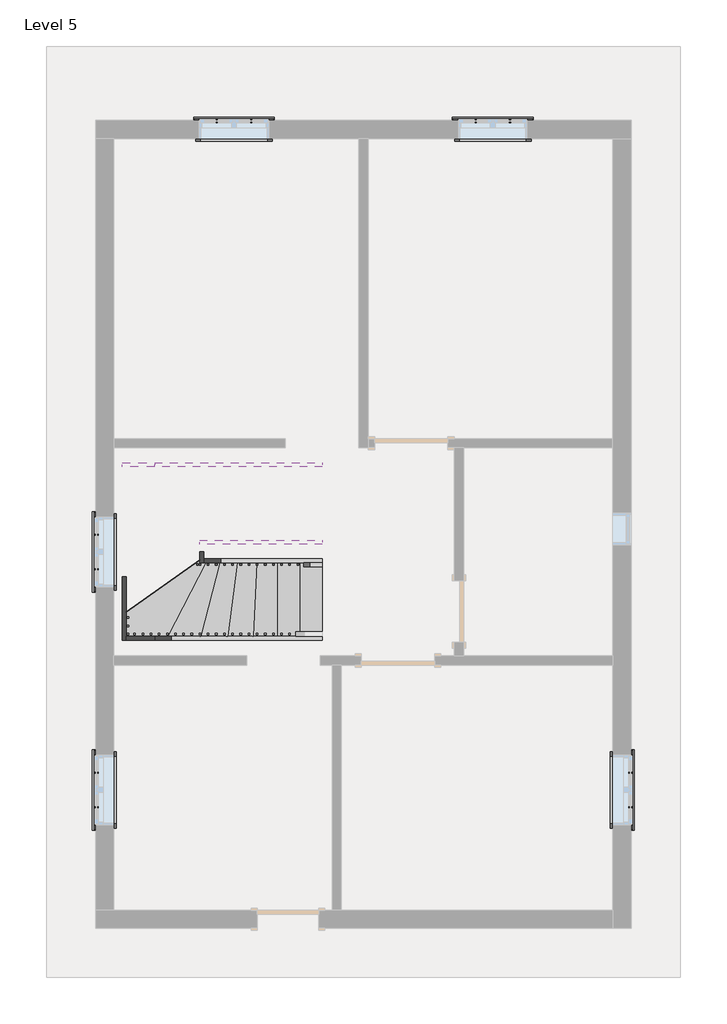
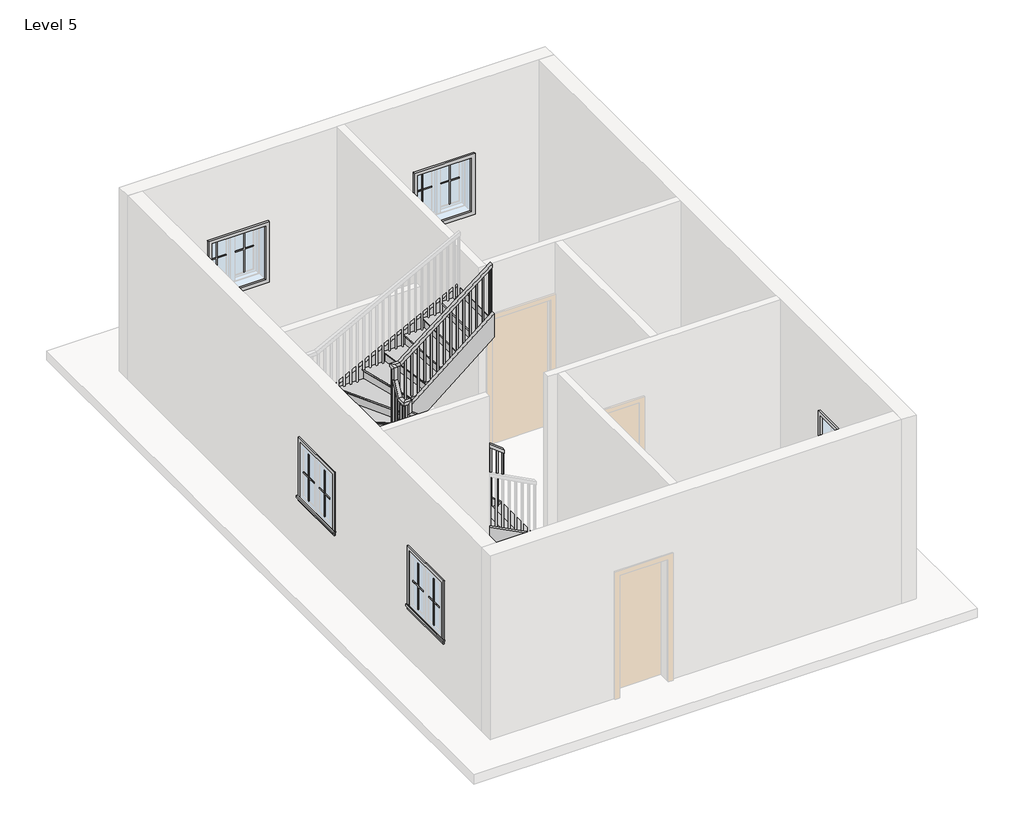
# One storey, part 2 of 2: 20 proxies, 8 members, 1 railing, 1 stair flight.
"""IFC4 building model written with IfcOpenShell, lengths in millimetres."""

from ifc_helpers import new_model, si_unit, frame, origin, place, context, project, spatial, polyline, outline, extrude, faceted_brep, transform, mapped, element, save
from components import muntin_pattern_2x2_muntin_pattern_2x2_b3fe6957, muntin_pattern_2x2_muntin_pattern_2x2_3e0ecaf2, trim_window_exterior_flat_with_sill_41619996, trim_window_interior_flat_picture_frame_51c85655, stair_flight_8889bdd5

model = new_model("IFC4")

# Units and contexts
model_context = context("Model", 3, world=origin())
ifc_project = project(units=[si_unit("LENGTHUNIT", "METRE", prefix="MILLI")], contexts=[model_context])

# Site, building, storey
site = spatial("IfcSite", under=ifc_project)
building = spatial("IfcBuilding", under=site)
storey = spatial("IfcBuildingStorey", under=building, Name="Level 5", Elevation=9601.2)

# Proxies
placement = place(None, origin())
muntin_pattern_2x2_muntin_pattern_2x2_shape = muntin_pattern_2x2_muntin_pattern_2x2_b3fe6957(model_context)
element("IfcBuildingElementProxy", 1, Name="Muntin Pattern_2x2 : Muntin Pattern_2x2", ObjectType="Muntin Pattern_2x2 : Muntin Pattern_2x2", at=placement, inside=storey, context=model_context, shape_type="MappedRepresentation", body=[
    mapped(muntin_pattern_2x2_muntin_pattern_2x2_shape, transform((-3096.8324167, 5150.2179147, 10585.45), x_axis=(1.0, 0.0, 0.0), y_axis=(0.0, 1.0, 0.0), z_axis=(0.0, 0.0, 1.0))),
])
element("IfcBuildingElementProxy", 2, Name="Muntin Pattern_2x2 : Muntin Pattern_2x2", ObjectType="Muntin Pattern_2x2 : Muntin Pattern_2x2", at=placement, inside=storey, context=model_context, shape_type="MappedRepresentation", body=[
    mapped(muntin_pattern_2x2_muntin_pattern_2x2_shape, transform((122.6175833, 5150.2179147, 10585.45), x_axis=(1.0, 0.0, 0.0), y_axis=(0.0, 1.0, 0.0), z_axis=(0.0, 0.0, 1.0))),
])
element("IfcBuildingElementProxy", 3, Name="Muntin Pattern_2x2 : Muntin Pattern_2x2", ObjectType="Muntin Pattern_2x2 : Muntin Pattern_2x2", at=placement, inside=storey, context=model_context, shape_type="MappedRepresentation", body=[
    mapped(muntin_pattern_2x2_muntin_pattern_2x2_shape, transform((2051.4300833, -2960.3195853, 10585.45), x_axis=(0.0, -1.0, 0.0), y_axis=(1.0, 0.0, 0.0), z_axis=(0.0, 0.0, 1.0))),
])
element("IfcBuildingElementProxy", 4, Name="Muntin Pattern_2x2 : Muntin Pattern_2x2", ObjectType="Muntin Pattern_2x2 : Muntin Pattern_2x2", at=placement, inside=storey, context=model_context, shape_type="MappedRepresentation", body=[
    mapped(muntin_pattern_2x2_muntin_pattern_2x2_shape, transform((-4597.0199167, -3388.9445853, 10585.45), x_axis=(0.0, 1.0, 0.0), y_axis=(-1.0, 0.0, 0.0), z_axis=(0.0, 0.0, 1.0))),
])
element("IfcBuildingElementProxy", 5, Name="Muntin Pattern_2x2 : Muntin Pattern_2x2", ObjectType="Muntin Pattern_2x2 : Muntin Pattern_2x2", at=placement, inside=storey, context=model_context, shape_type="MappedRepresentation", body=[
    mapped(muntin_pattern_2x2_muntin_pattern_2x2_shape, transform((-4597.0199167, -426.6695853, 10585.45), x_axis=(0.0, 1.0, 0.0), y_axis=(-1.0, 0.0, 0.0), z_axis=(0.0, 0.0, 1.0))),
])
muntin_pattern_2x2_muntin_pattern_2x2_2_shape = muntin_pattern_2x2_muntin_pattern_2x2_3e0ecaf2(model_context)
element("IfcBuildingElementProxy", 6, Name="Muntin Pattern_2x2 : Muntin Pattern_2x2", ObjectType="Muntin Pattern_2x2 : Muntin Pattern_2x2", at=placement, inside=storey, context=model_context, shape_type="MappedRepresentation", body=[
    mapped(muntin_pattern_2x2_muntin_pattern_2x2_2_shape, transform((-2668.2074167, 5150.2179147, 10585.45), x_axis=(-1.0, 0.0, 0.0), y_axis=(0.0, -1.0, 0.0), z_axis=(0.0, 0.0, 1.0))),
])
element("IfcBuildingElementProxy", 7, Name="Muntin Pattern_2x2 : Muntin Pattern_2x2", ObjectType="Muntin Pattern_2x2 : Muntin Pattern_2x2", at=placement, inside=storey, context=model_context, shape_type="MappedRepresentation", body=[
    mapped(muntin_pattern_2x2_muntin_pattern_2x2_2_shape, transform((551.2425833, 5150.2179147, 10585.45), x_axis=(-1.0, 0.0, 0.0), y_axis=(0.0, -1.0, 0.0), z_axis=(0.0, 0.0, 1.0))),
])
element("IfcBuildingElementProxy", 8, Name="Muntin Pattern_2x2 : Muntin Pattern_2x2", ObjectType="Muntin Pattern_2x2 : Muntin Pattern_2x2", at=placement, inside=storey, context=model_context, shape_type="MappedRepresentation", body=[
    mapped(muntin_pattern_2x2_muntin_pattern_2x2_2_shape, transform((2051.4300833, -3388.9445853, 10585.45), x_axis=(0.0, 1.0, 0.0), y_axis=(-1.0, 0.0, 0.0), z_axis=(0.0, 0.0, 1.0))),
])
element("IfcBuildingElementProxy", 9, Name="Muntin Pattern_2x2 : Muntin Pattern_2x2", ObjectType="Muntin Pattern_2x2 : Muntin Pattern_2x2", at=placement, inside=storey, context=model_context, shape_type="MappedRepresentation", body=[
    mapped(muntin_pattern_2x2_muntin_pattern_2x2_2_shape, transform((-4597.0199167, -2960.3195853, 10585.45), x_axis=(0.0, -1.0, 0.0), y_axis=(1.0, 0.0, 0.0), z_axis=(0.0, 0.0, 1.0))),
])
element("IfcBuildingElementProxy", 10, Name="Muntin Pattern_2x2 : Muntin Pattern_2x2", ObjectType="Muntin Pattern_2x2 : Muntin Pattern_2x2", at=placement, inside=storey, context=model_context, shape_type="MappedRepresentation", body=[
    mapped(muntin_pattern_2x2_muntin_pattern_2x2_2_shape, transform((-4597.0199167, 1.9554147, 10585.45), x_axis=(0.0, -1.0, 0.0), y_axis=(1.0, 0.0, 0.0), z_axis=(0.0, 0.0, 1.0))),
])
trim_window_exterior_flat_with_sill_shape = trim_window_exterior_flat_with_sill_41619996(model_context)
element("IfcBuildingElementProxy", 11, Name="Trim-Window-Exterior-Flat : with Sill", ObjectType="Trim-Window-Exterior-Flat : with Sill", at=placement, inside=storey, context=model_context, shape_type="MappedRepresentation", body=[
    mapped(trim_window_exterior_flat_with_sill_shape, transform((-2882.5199167, 5159.7429147, 11430.0), x_axis=(-1.0, 0.0, 0.0), y_axis=(0.0, 0.0, 1.0), z_axis=(0.0, 1.0, 0.0))),
])
element("IfcBuildingElementProxy", 12, Name="Trim-Window-Exterior-Flat : with Sill", ObjectType="Trim-Window-Exterior-Flat : with Sill", at=placement, inside=storey, context=model_context, shape_type="MappedRepresentation", body=[
    mapped(trim_window_exterior_flat_with_sill_shape, transform((336.9300833, 5159.7429147, 11430.0), x_axis=(-1.0, 0.0, 0.0), y_axis=(0.0, 0.0, 1.0), z_axis=(0.0, 1.0, 0.0))),
])
element("IfcBuildingElementProxy", 13, Name="Trim-Window-Exterior-Flat : with Sill", ObjectType="Trim-Window-Exterior-Flat : with Sill", at=placement, inside=storey, context=model_context, shape_type="MappedRepresentation", body=[
    mapped(trim_window_exterior_flat_with_sill_shape, transform((2060.9550833, -3174.6320853, 11430.0), x_axis=(0.0, 1.0, 0.0), y_axis=(0.0, 0.0, 1.0), z_axis=(1.0, 0.0, 0.0))),
])
element("IfcBuildingElementProxy", 14, Name="Trim-Window-Exterior-Flat : with Sill", ObjectType="Trim-Window-Exterior-Flat : with Sill", at=placement, inside=storey, context=model_context, shape_type="MappedRepresentation", body=[
    mapped(trim_window_exterior_flat_with_sill_shape, transform((-4606.5449167, -3174.6320853, 11430.0), x_axis=(0.0, -1.0, 0.0), y_axis=(0.0, 0.0, 1.0), z_axis=(-1.0, 0.0, 0.0))),
])
element("IfcBuildingElementProxy", 15, Name="Trim-Window-Exterior-Flat : with Sill", ObjectType="Trim-Window-Exterior-Flat : with Sill", at=placement, inside=storey, context=model_context, shape_type="MappedRepresentation", body=[
    mapped(trim_window_exterior_flat_with_sill_shape, transform((-4606.5449167, -212.3570853, 11430.0), x_axis=(0.0, -1.0, 0.0), y_axis=(0.0, 0.0, 1.0), z_axis=(-1.0, 0.0, 0.0))),
])
trim_window_interior_flat_picture_frame_shape = trim_window_interior_flat_picture_frame_51c85655(model_context)
element("IfcBuildingElementProxy", 16, Name="Trim-Window-Interior-Flat : Picture Frame", ObjectType="Trim-Window-Interior-Flat : Picture Frame", at=placement, inside=storey, context=model_context, shape_type="MappedRepresentation", body=[
    mapped(trim_window_interior_flat_picture_frame_shape, transform((-2882.5199167, 4931.1429147, 11430.0), x_axis=(1.0, 0.0, 0.0), y_axis=(0.0, 0.0, 1.0), z_axis=(0.0, -1.0, 0.0))),
])
element("IfcBuildingElementProxy", 17, Name="Trim-Window-Interior-Flat : Picture Frame", ObjectType="Trim-Window-Interior-Flat : Picture Frame", at=placement, inside=storey, context=model_context, shape_type="MappedRepresentation", body=[
    mapped(trim_window_interior_flat_picture_frame_shape, transform((336.9300833, 4931.1429147, 11430.0), x_axis=(1.0, 0.0, 0.0), y_axis=(0.0, 0.0, 1.0), z_axis=(0.0, -1.0, 0.0))),
])
element("IfcBuildingElementProxy", 18, Name="Trim-Window-Interior-Flat : Picture Frame", ObjectType="Trim-Window-Interior-Flat : Picture Frame", at=placement, inside=storey, context=model_context, shape_type="MappedRepresentation", body=[
    mapped(trim_window_interior_flat_picture_frame_shape, transform((1832.3550833, -3174.6320853, 11430.0), x_axis=(0.0, -1.0, 0.0), y_axis=(0.0, 0.0, 1.0), z_axis=(-1.0, 0.0, 0.0))),
])
element("IfcBuildingElementProxy", 19, Name="Trim-Window-Interior-Flat : Picture Frame", ObjectType="Trim-Window-Interior-Flat : Picture Frame", at=placement, inside=storey, context=model_context, shape_type="MappedRepresentation", body=[
    mapped(trim_window_interior_flat_picture_frame_shape, transform((-4377.9449167, -3174.6320853, 11430.0), x_axis=(0.0, 1.0, 0.0), y_axis=(0.0, 0.0, 1.0), z_axis=(1.0, 0.0, 0.0))),
])
element("IfcBuildingElementProxy", 20, Name="Trim-Window-Interior-Flat : Picture Frame", ObjectType="Trim-Window-Interior-Flat : Picture Frame", at=placement, inside=storey, context=model_context, shape_type="MappedRepresentation", body=[
    mapped(trim_window_interior_flat_picture_frame_shape, transform((-4377.9449167, -212.3570853, 11430.0), x_axis=(0.0, 1.0, 0.0), y_axis=(0.0, 0.0, 1.0), z_axis=(1.0, 0.0, 0.0))),
])

# Members
element("IfcMember", 21, ObjectType="Stringer - 2\" Width", at=placement, inside=storey, context=model_context, shape_type="SweptSolid", body=[
    extrude(outline(polyline([(9601.2, -1783.4132248), (9830.839954, -1783.4132248), (10906.5956453, -3870.8304165), (10563.700629, -3870.8304165), (9601.2, -2003.1755424), (9601.2, -1783.4132248)])), frame((0.0, -1310.9070853, 0.0), z_axis=(0.0, 1.0, 0.0), x_axis=(0.0, 0.0, 1.0)), (0.0, 0.0, 1.0), 50.8),
])
element("IfcMember", 22, ObjectType="Stringer - 2\" Width", at=placement, inside=storey, context=model_context, shape_type="SweptSolid", body=[
    extrude(outline(polyline([(-3870.8304165, -1260.1070853), (-3870.8304165, -1310.9070853), (-4225.5449167, -1310.9070853), (-4225.5449167, -1260.1070853), (-3870.8304165, -1260.1070853)])), frame((0.0, 0.0, 10563.700629), z_axis=(0.0, 0.0, 1.0), x_axis=(1.0, 0.0, 0.0)), (0.0, 0.0, 1.0), 342.8950162),
])
element("IfcMember", 23, ObjectType="Stringer - 2\" Width", at=placement, inside=storey, context=model_context, shape_type="SweptSolid", body=[
    extrude(outline(polyline([(-1310.9070853, 10601.7956453), (-1310.9070853, 10890.2952212), (811.1127974, 11571.1972697), (848.0929147, 11571.1972697), (848.0929147, 11240.1682298), (-1141.3846024, 10601.7956453), (-1310.9070853, 10601.7956453)])), frame((-4276.3449167, 0.0, 0.0), z_axis=(1.0, 0.0, 0.0), x_axis=(0.0, 1.0, 0.0)), (0.0, 0.0, 1.0), 50.8),
])
element("IfcMember", 24, ObjectType="Stringer - 2\" Width", at=placement, inside=storey, context=model_context, shape_type="SweptSolid", body=[
    extrude(outline(polyline([(-4276.3449167, 848.0929147), (-4276.3449167, 898.8929147), (-3870.8304165, 898.8929147), (-3870.8304165, 848.0929147), (-4276.3449167, 848.0929147)])), frame((0.0, 0.0, 11251.0904473), z_axis=(0.0, 0.0, 1.0), x_axis=(1.0, 0.0, 0.0)), (0.0, 0.0, 1.0), 320.1068224),
])
element("IfcMember", 25, ObjectType="Stringer - 2\" Width", at=placement, inside=storey, context=model_context, shape_type="SweptSolid", body=[
    extrude(outline(polyline([(11571.1972697, -3870.8304165), (11251.0904473, -3870.8304165), (12326.8461385, -1783.4132248), (12646.9529609, -1783.4132248), (11571.1972697, -3870.8304165)])), frame((0.0, 848.0929147, 0.0), z_axis=(0.0, 1.0, 0.0), x_axis=(0.0, 0.0, 1.0)), (0.0, 0.0, 1.0), 50.8),
])
element("IfcMember", 26, ObjectType="Stringer - 2\" Width", at=placement, inside=storey, context=model_context, shape_type="SweptSolid", body=[
    extrude(outline(polyline([(9601.2, -1783.4132248), (9777.3764461, -1783.4132248), (10981.618648, -3260.3449167), (10588.3410923, -3260.3449167), (9601.2, -2049.6748694), (9601.2, -1783.4132248)])), frame((0.0, -345.7070853, 0.0), z_axis=(0.0, 1.0, 0.0), x_axis=(0.0, 0.0, 1.0)), (0.0, 0.0, 1.0), 50.8),
])
element("IfcMember", 27, ObjectType="Stringer - 2\" Width", at=placement, inside=storey, context=model_context, shape_type="SweptSolid", body=[
    extrude(outline(polyline([(-345.7070853, 10629.7617647), (-345.7070853, 11174.4682978), (-139.0699679, 11527.3409689), (-117.1070853, 11527.3409689), (-117.1070853, 10961.665107), (-311.464868, 10629.7617647), (-345.7070853, 10629.7617647)])), frame((-3311.1449167, 0.0, 0.0), z_axis=(1.0, 0.0, 0.0), x_axis=(0.0, 1.0, 0.0)), (0.0, 0.0, 1.0), 50.8),
])
element("IfcMember", 28, ObjectType="Stringer - 2\" Width", at=placement, inside=storey, context=model_context, shape_type="SweptSolid", body=[
    extrude(outline(polyline([(11527.3409689, -3311.1449167), (11134.0634131, -3311.1449167), (12379.7262875, -1783.4132248), (12773.0038432, -1783.4132248), (11527.3409689, -3311.1449167)])), frame((0.0, -117.1070853, 0.0), z_axis=(0.0, 1.0, 0.0), x_axis=(0.0, 0.0, 1.0)), (0.0, 0.0, 1.0), 50.8),
])

# Railing
element("IfcRailing", 29, ObjectType="Handrail - Rectangular", at=placement, inside=storey, context=model_context, shape_type="SolidModel", body=[
    faceted_brep([(-1783.4132248, -396.5070853, 10684.9333333), (-1783.4132248, -396.5070853, 10620.6000346), (-1783.4132248, -345.7070853, 10620.6000346), (-1783.4132248, -345.7070853, 10684.9333333), (-3234.9449167, -396.5070853, 11812.8191036), (-3285.7449167, -396.5070853, 11787.9590024), (-3285.7449167, -345.7070853, 11787.9590024), (-3234.9449167, -345.7070853, 11812.8191036), (-3234.9449167, -396.5070853, 12015.8281882), (-3285.7449167, -396.5070853, 11965.0281882), (-3285.7449167, -345.7070853, 11965.0281882), (-3234.9449167, -345.7070853, 12015.8281882), (-3361.9449167, -396.5070853, 12015.8281882), (-3361.9449167, -396.5070853, 11965.0281882), (-3311.1449167, -345.7070853, 11965.0281882), (-3311.1449167, -345.7070853, 12015.8281882), (-3361.9449167, -269.5070853, 12015.8281882), (-3361.9449167, -240.3857515, 11965.0281882), (-3311.1449167, -240.3857515, 11965.0281882), (-3311.1449167, -269.5070853, 12015.8281882), (-3361.9449167, -142.5070853, 12232.7051451), (-3361.9449167, -91.7070853, 12218.9256424), (-3311.1449167, -91.7070853, 12218.9256424), (-3311.1449167, -142.5070853, 12232.7051451), (-3361.9449167, -142.5070853, 12435.7142297), (-3361.9449167, -91.7070853, 12384.9142297), (-3311.1449167, -91.7070853, 12384.9142297), (-3311.1449167, -142.5070853, 12435.7142297), (-3361.9449167, -15.5070853, 12435.7142297), (-3361.9449167, -15.5070853, 12384.9142297), (-3311.1449167, -66.3070853, 12384.9142297), (-3311.1449167, -66.3070853, 12435.7142297), (-3234.9449167, -15.5070853, 12435.7142297), (-3217.5282487, -15.5070853, 12384.9142297), (-3217.5282487, -66.3070853, 12384.9142297), (-3234.9449167, -66.3070853, 12435.7142297), (-1783.4132248, -15.5070853, 13563.6), (-1783.4132248, -66.3070853, 13563.6), (-1783.4132248, -66.3070853, 13499.2667013), (-1783.4132248, -15.5070853, 13499.2667013)], [[[0, 1, 2, 3]], [[1, 0, 4, 5]], [[2, 1, 5, 6]], [[3, 2, 6, 7]], [[0, 3, 7, 4]], [[5, 4, 8, 9]], [[6, 5, 9, 10]], [[7, 6, 10, 11]], [[4, 7, 11, 8]], [[9, 8, 12, 13]], [[10, 9, 13, 14]], [[11, 10, 14, 15]], [[8, 11, 15, 12]], [[13, 12, 16, 17]], [[14, 13, 17, 18]], [[15, 14, 18, 19]], [[12, 15, 19, 16]], [[17, 16, 20, 21]], [[18, 17, 21, 22]], [[19, 18, 22, 23]], [[16, 19, 23, 20]], [[21, 20, 24, 25]], [[22, 21, 25, 26]], [[23, 22, 26, 27]], [[20, 23, 27, 24]], [[25, 24, 28, 29]], [[26, 25, 29, 30]], [[27, 26, 30, 31]], [[24, 27, 31, 28]], [[29, 28, 32, 33]], [[30, 29, 33, 34]], [[31, 30, 34, 35]], [[28, 31, 35, 32]], [[36, 37, 38, 39]], [[33, 32, 36, 39]], [[34, 33, 39, 38]], [[35, 34, 38, 37]], [[32, 35, 37, 36]]]),
    extrude(outline(polyline([(13484.0316852, -1803.0199167), (13469.2292361, -1822.0699167), (12479.8666667, -1822.0699167), (12479.8666667, -1803.0199167), (13484.0316852, -1803.0199167)])), frame((0.0, -50.4320853, 0.0), z_axis=(0.0, 1.0, 0.0), x_axis=(0.0, 0.0, 1.0)), (0.0, 0.0, 1.0), 19.05),
    extrude(outline(polyline([(13405.0852902, -1904.6199167), (13390.2828411, -1923.6699167), (12479.8666667, -1923.6699167), (12479.8666667, -1904.6199167), (13405.0852902, -1904.6199167)])), frame((0.0, -50.4320853, 0.0), z_axis=(0.0, 1.0, 0.0), x_axis=(0.0, 0.0, 1.0)), (0.0, 0.0, 1.0), 19.05),
    extrude(outline(polyline([(13326.1388952, -2006.2199167), (13311.3364462, -2025.2699167), (12479.8666667, -2025.2699167), (12479.8666667, -2006.2199167), (13326.1388952, -2006.2199167)])), frame((0.0, -50.4320853, 0.0), z_axis=(0.0, 1.0, 0.0), x_axis=(0.0, 0.0, 1.0)), (0.0, 0.0, 1.0), 19.05),
    extrude(outline(polyline([(13247.1925003, -2107.8199167), (13232.3900512, -2126.8699167), (12310.5333333, -2126.8699167), (12310.5333333, -2107.8199167), (13247.1925003, -2107.8199167)])), frame((0.0, -50.4320853, 0.0), z_axis=(0.0, 1.0, 0.0), x_axis=(0.0, 0.0, 1.0)), (0.0, 0.0, 1.0), 19.05),
    extrude(outline(polyline([(13168.2461053, -2209.4199167), (13153.4436562, -2228.4699167), (12310.5333333, -2228.4699167), (12310.5333333, -2209.4199167), (13168.2461053, -2209.4199167)])), frame((0.0, -50.4320853, 0.0), z_axis=(0.0, 1.0, 0.0), x_axis=(0.0, 0.0, 1.0)), (0.0, 0.0, 1.0), 19.05),
    extrude(outline(polyline([(13089.2997103, -2311.0199167), (13074.4972613, -2330.0699167), (12310.5333333, -2330.0699167), (12310.5333333, -2311.0199167), (13089.2997103, -2311.0199167)])), frame((0.0, -50.4320853, 0.0), z_axis=(0.0, 1.0, 0.0), x_axis=(0.0, 0.0, 1.0)), (0.0, 0.0, 1.0), 19.05),
    extrude(outline(polyline([(13010.3533154, -2412.6199167), (12995.5508663, -2431.6699167), (12141.2, -2431.6699167), (12141.2, -2412.6199167), (13010.3533154, -2412.6199167)])), frame((0.0, -50.4320853, 0.0), z_axis=(0.0, 1.0, 0.0), x_axis=(0.0, 0.0, 1.0)), (0.0, 0.0, 1.0), 19.05),
    extrude(outline(polyline([(12931.4069204, -2514.2199167), (12916.6044713, -2533.2699167), (12141.2, -2533.2699167), (12141.2, -2514.2199167), (12931.4069204, -2514.2199167)])), frame((0.0, -50.4320853, 0.0), z_axis=(0.0, 1.0, 0.0), x_axis=(0.0, 0.0, 1.0)), (0.0, 0.0, 1.0), 19.05),
    extrude(outline(polyline([(12852.4605254, -2615.8199167), (12837.6580764, -2634.8699167), (11971.8666667, -2634.8699167), (11971.8666667, -2615.8199167), (12852.4605254, -2615.8199167)])), frame((0.0, -50.4320853, 0.0), z_axis=(0.0, 1.0, 0.0), x_axis=(0.0, 0.0, 1.0)), (0.0, 0.0, 1.0), 19.05),
    extrude(outline(polyline([(12773.5141304, -2717.4199167), (12758.7116814, -2736.4699167), (11971.8666667, -2736.4699167), (11971.8666667, -2717.4199167), (12773.5141304, -2717.4199167)])), frame((0.0, -50.4320853, 0.0), z_axis=(0.0, 1.0, 0.0), x_axis=(0.0, 0.0, 1.0)), (0.0, 0.0, 1.0), 19.05),
    extrude(outline(polyline([(12694.5677355, -2819.0199167), (12679.7652864, -2838.0699167), (11971.8666667, -2838.0699167), (11971.8666667, -2819.0199167), (12694.5677355, -2819.0199167)])), frame((0.0, -50.4320853, 0.0), z_axis=(0.0, 1.0, 0.0), x_axis=(0.0, 0.0, 1.0)), (0.0, 0.0, 1.0), 19.05),
    extrude(outline(polyline([(12615.6213405, -2920.6199167), (12600.8188914, -2939.6699167), (11802.5333333, -2939.6699167), (11802.5333333, -2920.6199167), (12615.6213405, -2920.6199167)])), frame((0.0, -50.4320853, 0.0), z_axis=(0.0, 1.0, 0.0), x_axis=(0.0, 0.0, 1.0)), (0.0, 0.0, 1.0), 19.05),
    extrude(outline(polyline([(12536.6749455, -3022.2199167), (12521.8724965, -3041.2699167), (11802.5333333, -3041.2699167), (11802.5333333, -3022.2199167), (12536.6749455, -3022.2199167)])), frame((0.0, -50.4320853, 0.0), z_axis=(0.0, 1.0, 0.0), x_axis=(0.0, 0.0, 1.0)), (0.0, 0.0, 1.0), 19.05),
    extrude(outline(polyline([(12457.7285506, -3123.8199167), (12442.9261015, -3142.8699167), (11633.2, -3142.8699167), (11633.2, -3123.8199167), (12457.7285506, -3123.8199167)])), frame((0.0, -50.4320853, 0.0), z_axis=(0.0, 1.0, 0.0), x_axis=(0.0, 0.0, 1.0)), (0.0, 0.0, 1.0), 19.05),
    extrude(outline(polyline([(12378.7821556, -3225.4199167), (12363.9797065, -3244.4699167), (11633.2, -3244.4699167), (11633.2, -3225.4199167), (12378.7821556, -3225.4199167)])), frame((0.0, -50.4320853, 0.0), z_axis=(0.0, 1.0, 0.0), x_axis=(0.0, 0.0, 1.0)), (0.0, 0.0, 1.0), 19.05),
    extrude(outline(polyline([(-3327.0199167, -75.8320853), (-3346.0699167, -75.8320853), (-3346.0699167, -56.7820853), (-3327.0199167, -56.7820853), (-3327.0199167, -75.8320853)])), frame((0.0, 0.0, 11294.5333333), z_axis=(0.0, 0.0, 1.0), x_axis=(1.0, 0.0, 0.0)), (0.0, 0.0, 1.0), 1090.3808964),
    extrude(outline(polyline([(-177.4320853, 12072.5336964), (-158.3820853, 12105.06524), (-158.3820853, 11125.2), (-177.4320853, 11125.2), (-177.4320853, 12072.5336964)])), frame((-3346.0699167, 0.0, 0.0), z_axis=(1.0, 0.0, 0.0), x_axis=(0.0, 1.0, 0.0)), (0.0, 0.0, 1.0), 19.05),
    extrude(outline(polyline([(-279.0320853, 11899.0321309), (-259.9820853, 11931.5636744), (-259.9820853, 10955.8666667), (-279.0320853, 10955.8666667), (-279.0320853, 11899.0321309)])), frame((-3346.0699167, 0.0, 0.0), z_axis=(1.0, 0.0, 0.0), x_axis=(0.0, 1.0, 0.0)), (0.0, 0.0, 1.0), 19.05),
    extrude(outline(polyline([(-3297.8882248, -361.5820853), (-3297.8882248, -380.6320853), (-3316.9382248, -380.6320853), (-3316.9382248, -361.5820853), (-3297.8882248, -361.5820853)])), frame((0.0, 0.0, 10786.5333333), z_axis=(0.0, 0.0, 1.0), x_axis=(1.0, 0.0, 0.0)), (0.0, 0.0, 1.0), 1178.4948549),
    extrude(outline(polyline([(11718.4483397, -3196.2882248), (11733.2507888, -3215.3382248), (10617.2, -3215.3382248), (10617.2, -3196.2882248), (11718.4483397, -3196.2882248)])), frame((0.0, -380.6320853, 0.0), z_axis=(0.0, 1.0, 0.0), x_axis=(0.0, 0.0, 1.0)), (0.0, 0.0, 1.0), 19.05),
    extrude(outline(polyline([(11639.5019447, -3094.6882248), (11654.3043938, -3113.7382248), (10617.2, -3113.7382248), (10617.2, -3094.6882248), (11639.5019447, -3094.6882248)])), frame((0.0, -380.6320853, 0.0), z_axis=(0.0, 1.0, 0.0), x_axis=(0.0, 0.0, 1.0)), (0.0, 0.0, 1.0), 19.05),
    extrude(outline(polyline([(11560.5555498, -2993.0882248), (11575.3579988, -3012.1382248), (10447.8666667, -3012.1382248), (10447.8666667, -2993.0882248), (11560.5555498, -2993.0882248)])), frame((0.0, -380.6320853, 0.0), z_axis=(0.0, 1.0, 0.0), x_axis=(0.0, 0.0, 1.0)), (0.0, 0.0, 1.0), 19.05),
    extrude(outline(polyline([(11481.6091548, -2891.4882248), (11496.4116039, -2910.5382248), (10447.8666667, -2910.5382248), (10447.8666667, -2891.4882248), (11481.6091548, -2891.4882248)])), frame((0.0, -380.6320853, 0.0), z_axis=(0.0, 1.0, 0.0), x_axis=(0.0, 0.0, 1.0)), (0.0, 0.0, 1.0), 19.05),
    extrude(outline(polyline([(11402.6627598, -2789.8882248), (11417.4652089, -2808.9382248), (10278.5333333, -2808.9382248), (10278.5333333, -2789.8882248), (11402.6627598, -2789.8882248)])), frame((0.0, -380.6320853, 0.0), z_axis=(0.0, 1.0, 0.0), x_axis=(0.0, 0.0, 1.0)), (0.0, 0.0, 1.0), 19.05),
    extrude(outline(polyline([(11323.7163649, -2688.2882248), (11338.5188139, -2707.3382248), (10278.5333333, -2707.3382248), (10278.5333333, -2688.2882248), (11323.7163649, -2688.2882248)])), frame((0.0, -380.6320853, 0.0), z_axis=(0.0, 1.0, 0.0), x_axis=(0.0, 0.0, 1.0)), (0.0, 0.0, 1.0), 19.05),
    extrude(outline(polyline([(11244.7699699, -2586.6882248), (11259.5724189, -2605.7382248), (10109.2, -2605.7382248), (10109.2, -2586.6882248), (11244.7699699, -2586.6882248)])), frame((0.0, -380.6320853, 0.0), z_axis=(0.0, 1.0, 0.0), x_axis=(0.0, 0.0, 1.0)), (0.0, 0.0, 1.0), 19.05),
    extrude(outline(polyline([(11165.8235749, -2485.0882248), (11180.626024, -2504.1382248), (10109.2, -2504.1382248), (10109.2, -2485.0882248), (11165.8235749, -2485.0882248)])), frame((0.0, -380.6320853, 0.0), z_axis=(0.0, 1.0, 0.0), x_axis=(0.0, 0.0, 1.0)), (0.0, 0.0, 1.0), 19.05),
    extrude(outline(polyline([(11086.8771799, -2383.4882248), (11101.679629, -2402.5382248), (10109.2, -2402.5382248), (10109.2, -2383.4882248), (11086.8771799, -2383.4882248)])), frame((0.0, -380.6320853, 0.0), z_axis=(0.0, 1.0, 0.0), x_axis=(0.0, 0.0, 1.0)), (0.0, 0.0, 1.0), 19.05),
    extrude(outline(polyline([(11007.930785, -2281.8882248), (11022.733234, -2300.9382248), (9939.8666667, -2300.9382248), (9939.8666667, -2281.8882248), (11007.930785, -2281.8882248)])), frame((0.0, -380.6320853, 0.0), z_axis=(0.0, 1.0, 0.0), x_axis=(0.0, 0.0, 1.0)), (0.0, 0.0, 1.0), 19.05),
    extrude(outline(polyline([(10928.98439, -2180.2882248), (10943.7868391, -2199.3382248), (9939.8666667, -2199.3382248), (9939.8666667, -2180.2882248), (10928.98439, -2180.2882248)])), frame((0.0, -380.6320853, 0.0), z_axis=(0.0, 1.0, 0.0), x_axis=(0.0, 0.0, 1.0)), (0.0, 0.0, 1.0), 19.05),
    extrude(outline(polyline([(10850.037995, -2078.6882248), (10864.8404441, -2097.7382248), (9939.8666667, -2097.7382248), (9939.8666667, -2078.6882248), (10850.037995, -2078.6882248)])), frame((0.0, -380.6320853, 0.0), z_axis=(0.0, 1.0, 0.0), x_axis=(0.0, 0.0, 1.0)), (0.0, 0.0, 1.0), 19.05),
    extrude(outline(polyline([(10771.0916001, -1977.0882248), (10785.8940491, -1996.1382248), (9770.5333333, -1996.1382248), (9770.5333333, -1977.0882248), (10771.0916001, -1977.0882248)])), frame((0.0, -380.6320853, 0.0), z_axis=(0.0, 1.0, 0.0), x_axis=(0.0, 0.0, 1.0)), (0.0, 0.0, 1.0), 19.05),
    extrude(outline(polyline([(10692.1452051, -1875.4882248), (10706.9476541, -1894.5382248), (9770.5333333, -1894.5382248), (9770.5333333, -1875.4882248), (10692.1452051, -1875.4882248)])), frame((0.0, -380.6320853, 0.0), z_axis=(0.0, 1.0, 0.0), x_axis=(0.0, 0.0, 1.0)), (0.0, 0.0, 1.0), 19.05),
    extrude(outline(polyline([(-3327.0199167, -50.4320853), (-3346.0699167, -50.4320853), (-3346.0699167, -31.3820853), (-3327.0199167, -31.3820853), (-3327.0199167, -50.4320853)])), frame((0.0, 0.0, 11463.8666667), z_axis=(0.0, 0.0, 1.0), x_axis=(1.0, 0.0, 0.0)), (0.0, 0.0, 1.0), 921.0475631),
    extrude(outline(polyline([(-3327.0199167, -361.5820853), (-3327.0199167, -380.6320853), (-3346.0699167, -380.6320853), (-3346.0699167, -361.5820853), (-3327.0199167, -361.5820853)])), frame((0.0, 0.0, 10786.5333333), z_axis=(0.0, 0.0, 1.0), x_axis=(1.0, 0.0, 0.0)), (0.0, 0.0, 1.0), 1178.4948549),
    extrude(outline(polyline([(13499.2667013, -1783.4132248), (13484.4642523, -1802.4632248), (12479.8666667, -1802.4632248), (12479.8666667, -1783.4132248), (13499.2667013, -1783.4132248)])), frame((0.0, -50.4320853, 0.0), z_axis=(0.0, 1.0, 0.0), x_axis=(0.0, 0.0, 1.0)), (0.0, 0.0, 1.0), 19.05),
    extrude(outline(polyline([(10620.6000346, -1783.4132248), (10635.4024837, -1802.4632248), (9770.5333333, -1802.4632248), (9770.5333333, -1783.4132248), (10620.6000346, -1783.4132248)])), frame((0.0, -380.6320853, 0.0), z_axis=(0.0, 1.0, 0.0), x_axis=(0.0, 0.0, 1.0)), (0.0, 0.0, 1.0), 19.05),
])

# Stair flight
stair_flight_shape = stair_flight_8889bdd5(model_context)
element("IfcStairFlight", 30, ObjectType="2\" Tread 1\" Nosing 1/4\" Riser", at=placement, inside=storey, context=model_context, shape_type="MappedRepresentation", body=[
    mapped(stair_flight_shape, transform((0.0, 0.0, 0.0), x_axis=(1.0, 0.0, 0.0), y_axis=(0.0, 1.0, 0.0), z_axis=(0.0, 0.0, 1.0))),
])

save(model, "model.ifc")

# Revit data of these elements
# Type "Muntin Pattern_2x2 : Muntin Pattern_2x2"
#   Width [instance default] = 4' - 0"
#   Thickness = 0' - 0 1/2"
#   Height [instance default] = 4' - 0"
#   Distance = 0' - 0 3/4"
#   Interior Material [instance default] = none
#   Exterior Material [instance default] = none
#   Default Elevation = 0
# Type "Trim-Window-Exterior-Flat : with Sill"
#   Trim Width = 0' - 2 1/4"
#   Trim Thickness_Picture Frame = 0' - 1 1/4"
#   Trim Thickness_with Sill = 0' - 0 3/4"
#   Sill Thickness = 0' - 1 1/4"
#   Opening Width [instance default] = 2' - 0"
#   Opening Height [instance default] = 3' - 0"
#   Default Elevation = 4' - 0"
#   Sill = yes
#   Picture Frame = no
#   Trim Material [instance default] = none
# Type "Trim-Window-Interior-Flat : Picture Frame"
#   Trim Thickness_Picture Frame = 0' - 1 1/4"
#   Trim Width = 0' - 2 1/4"
#   Trim Thickness_with Sill = 0' - 0 3/4"
#   Sill Thickness = 0' - 1 1/4"
#   Opening Width [instance default] = 2' - 0"
#   Opening Height [instance default] = 3' - 0"
#   Default Elevation = 4' - 0"
#   Sill = no
#   Picture Frame = yes
#   Trim Material [instance default] = none
# Type "Handrail - Rectangular"
#   Assembly Code = "C2010400"
#   built-in parameter 1008612 = 0.0416667 (stored number, unit not read)
#   built-in parameter 1008611 = 0.0416667 (stored number, unit not read)
#   built-in parameter 1008609 = 0.333333 (stored number, unit not read)
#   built-in parameter 1008604 = 0.166667 (stored number, unit not read)
#   built-in parameter 1008603 = 0.166667 (stored number, unit not read)
#   Railing Height = 3' - 0"
#   built-in parameter 1008630 = 2
#   built-in parameter 1008610 = 2
#   built-in parameter 1008618 = Baluster - Square : 3/4"
# Elements 1, 2, 3, 4, 5, 6, 7, 8, 9, 10 (IfcBuildingElementProxy, "Muntin Pattern_2x2 : Muntin Pattern_2x2")
#   Width = 0' - 11 5/8"
#   Height = 2' - 6 1/2"
#   Interior Material = Wood - Stained
#   Exterior Material = Clad - White
#   Phase Created = New Construction
#   Materials on its faces: "Clad - White", "Wood - Stained"
# Elements 11, 12, 13, 14, 15 (IfcBuildingElementProxy, "Trim-Window-Exterior-Flat : with Sill")
#   Opening Width = 2' - 10"
#   Opening Height = 3' - 0"
#   Trim Material = Clad - White
#   Phase Created = New Construction
#   Materials on its faces: "Clad - White"
# Elements 16, 17, 18, 19, 20 (IfcBuildingElementProxy, "Trim-Window-Interior-Flat : Picture Frame")
#   Opening Width = 2' - 10"
#   Opening Height = 3' - 0"
#   Trim Material = Wood - Stained
#   Phase Created = New Construction
#   Materials on its faces: "Wood - Stained"
# Elements 21, 22, 23, 24, 25, 26, 27, 28 (IfcMember, "Stringer - 2\" Width")
#   Phase Created = New Construction
# Element 29 (IfcRailing, "Handrail - Rectangular")
#   Phase Created = New Construction
# Element 30 (IfcStairFlight, "2\" Tread 1\" Nosing 1/4\" Riser")
#   Phase Created = New Construction
# Materials
#   "Clad - White": class "Wood", colour RGB 242 242 238, transparency 0, Cost = 0
#   "Wood - Stained": class "Wood", colour RGB 224 178 126, transparency 0, Cost = 0
